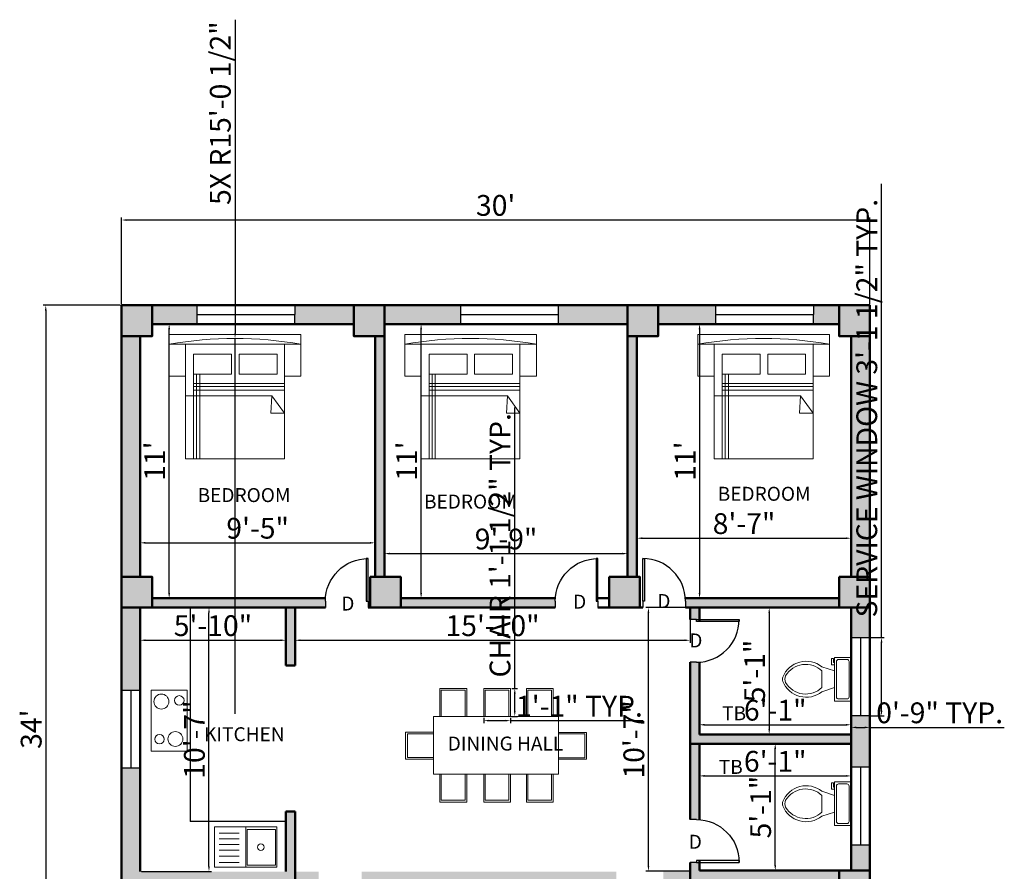
# Model space of a CAD drawing. Units: inches. Extents: x 1864 to 2337, y 2028 to 2650.
# Tile 2 of 2: x 1864 to 2337, y 2240 to 2650. Entities that reach past the tile are written whole.
import ezdxf

# ---------------------------------------------------------------- set-up
doc = ezdxf.new("R2010")
doc.units = ezdxf.units.IN
for name, color, linetype, lineweight in [('A-ANNO-TEXT', 7, 'Continuous', 25), ('A-AREA-IDEN', 7, 'Continuous', 25), ('A-COLS-PATT', 10, 'Continuous', 13), ('A-EQPM', 93, 'Continuous', 18), ('A-FLOR-CASE', 7, 'Continuous', 25), ('A-FLOR-FIXT', 93, 'Continuous', 18), ('A-WALL-PATT', 144, 'Continuous', 13), ('BED', 220, 'Continuous', 18), ('COLUMN', 10, 'Continuous', 50), ('DIM', 130, 'Continuous', 18), ('WALL', 7, 'Continuous', 50)]:
    doc.layers.add(name, color=color, linetype=linetype, lineweight=lineweight)
for name, color, linetype, lineweight, plot in [('DINING', 11, 'Continuous', 18, False), ('DOOR', 50, 'Continuous', 25, False), ('WINDOW', 244, 'Continuous', 25, False)]:
    doc.layers.add(name, color=color, linetype=linetype, lineweight=lineweight, plot=plot)
doc.styles.get("Standard").update_dxf_attribs({"font": 'arial.ttf'})
doc.dimstyles.new('ISO-25', dxfattribs={"dimtxt": 10, "dimasz": 2.5, "dimexe": 1.25, "dimexo": 0.625, "dimtad": 1, "dimdec": 0, "dimlunit": 4, "dimtxsty": 'Standard', "dimcen": 2.5, "dimadec": 0, "dimazin": 0, "dimtfac": 1, "dimtdec": 0, "dimtmove": 0, "dimatfit": 3, "dimfxl": 1, "dimarcsym": 0})

# ---------------------------------------------------------------- blocks, each defined once
blk = doc.blocks.new('*U4')
for p, q in [((9.5, -6), (9.5, -2)), ((-10, -8.5), (-8, -8.5)), ((-10, -9.5), (-10, -8.5)), ((-8, -8.5), (-8, -8)), ((-7, -8), (-7, -9.5)), ((-4, -8), (-6, -14)), ((4, -8), (6, -14)), ((-7, -9.5), (-10, -9.5)), ((4, -14), (-4, -14))]:
    blk.add_line(p, q)
blk.add_lwpolyline([(10.5, -8), (10.5, 0), (-10.5, 0), (-10.5, -8)], close=True)
for points in [[(-9.5, -2), (-9.5, -6)], [(8.5, -1), (-8.5, -1)], [(-8.5, -7), (8.5, -7)]]:
    blk.add_lwpolyline(points)
for centre, radius, start, end in [((-8.62, -1.88), 0.884, 81.8699, 188.1301), ((8.62, -1.88), 0.884, 351.8699, 98.1301), ((-8.62, -6.12), 0.884, 171.8699, 278.1301), ((8.62, -6.12), 0.884, 261.8699, 8.1301), ((3.52, -21.58), 12.17, 141.4691, 247.9714), ((4.2, -21.82), 11.33, 136.3677, 238.9468), ((-3.52, -21.58), 12.17, 292.0284, 38.5307), ((-4.2, -21.82), 11.33, 301.053, 43.6321), ((0, -27.88), 4, 245.7318, 294.2682), ((0, -29), 4, 254.8605, 285.1395)]:
    blk.add_arc(centre, radius, start, end)
blk = doc.blocks.new('*U2')
for p, q in [((0, 0), (0, -6)), ((40, 0), (40, -6))]:
    blk.add_line(p, q)
blk.add_lwpolyline([(0, 0), (0, 40), (1.75, 40), (1.75, 0)], close=True)
blk.add_arc((0, 0), 40, 0, 90)
blk = doc.blocks.new('*D5')
at = {"layer": 'Defpoints', "color": 0, "transparency": 16777216}
for p in [(1921.75, 2497.33), (2034.75, 2497.33), (2034.75, 2397.81)]:
    blk.add_point(p, dxfattribs=at)
at = {"layer": 'DIM', "color": 0, "lineweight": -2, "transparency": 16777216}
for p, q in [((1921.75, 2496.7), (1921.75, 2396.56)), ((2034.75, 2496.7), (2034.75, 2396.56)), ((1924.25, 2397.81), (2032.25, 2397.81))]:
    blk.add_line(p, q, dxfattribs=at)
at = {"layer": 'DIM', "color": 0, "transparency": 16777216}
for points in [[(1924.25, 2398.23), (1924.25, 2397.4), (1921.75, 2397.81)], [(2032.25, 2398.23), (2032.25, 2397.4), (2034.75, 2397.81)]]:
    blk.add_solid(points, dxfattribs=at)
at = {"layer": 'DIM', "color": 0, "transparency": 16777216, "insert": (1978.25, 2403.54), "char_height": 10, "attachment_point": 5}
blk.add_mtext('9\'-5"', dxfattribs=at)
blk = doc.blocks.new('*D6')
at = {"layer": 'Defpoints', "color": 0, "transparency": 16777216}
for p in [(1927.51, 2503.12), (1935.69, 2503.12), (1927.51, 2371.12)]:
    blk.add_point(p, dxfattribs=at)
at = {"layer": 'DIM', "color": 0, "lineweight": -2, "transparency": 16777216}
for p, q in [((1928.14, 2503.12), (1936.94, 2503.12)), ((1935.69, 2373.62), (1935.69, 2500.62)), ((1928.14, 2371.12), (1936.94, 2371.12))]:
    blk.add_line(p, q, dxfattribs=at)
at = {"layer": 'DIM', "color": 0, "transparency": 16777216}
for points in [[(1935.27, 2500.62), (1936.11, 2500.62), (1935.69, 2503.12)], [(1935.27, 2373.62), (1936.11, 2373.62), (1935.69, 2371.12)]]:
    blk.add_solid(points, dxfattribs=at)
at = {"layer": 'DIM', "color": 0, "transparency": 16777216, "insert": (1930.04, 2437.12), "char_height": 10, "attachment_point": 5, "rotation": 90}
blk.add_mtext("11'", dxfattribs=at)
blk = doc.blocks.new('*D7')
at = {"layer": 'Defpoints', "color": 0, "transparency": 16777216}
for p in [(2039.25, 2503.12), (2056.9, 2503.12), (2047.12, 2371.12)]:
    blk.add_point(p, dxfattribs=at)
at = {"layer": 'DIM', "color": 0, "lineweight": -2, "transparency": 16777216}
for p, q in [((2039.88, 2503.12), (2058.15, 2503.12)), ((2056.9, 2373.62), (2056.9, 2500.62)), ((2047.75, 2371.12), (2058.15, 2371.12))]:
    blk.add_line(p, q, dxfattribs=at)
at = {"layer": 'DIM', "color": 0, "transparency": 16777216}
for points in [[(2056.48, 2500.62), (2057.32, 2500.62), (2056.9, 2503.12)], [(2056.48, 2373.62), (2057.32, 2373.62), (2056.9, 2371.12)]]:
    blk.add_solid(points, dxfattribs=at)
at = {"layer": 'DIM', "color": 0, "transparency": 16777216, "insert": (2051.25, 2437.12), "char_height": 10, "attachment_point": 5, "rotation": 90}
blk.add_mtext("11'", dxfattribs=at)
blk = doc.blocks.new('*D8')
at = {"layer": 'Defpoints', "color": 0, "transparency": 16777216}
for p in [(2156.25, 2392.62), (2039.25, 2381.41), (2156.25, 2381.41)]:
    blk.add_point(p, dxfattribs=at)
at = {"layer": 'DIM', "color": 0, "lineweight": -2, "transparency": 16777216}
for p, q in [((2039.25, 2382.03), (2039.25, 2393.87)), ((2041.75, 2392.62), (2153.75, 2392.62)), ((2156.25, 2382.03), (2156.25, 2393.87))]:
    blk.add_line(p, q, dxfattribs=at)
at = {"layer": 'DIM', "color": 0, "transparency": 16777216}
for points in [[(2041.75, 2393.04), (2041.75, 2392.21), (2039.25, 2392.62)], [(2153.75, 2393.04), (2153.75, 2392.21), (2156.25, 2392.62)]]:
    blk.add_solid(points, dxfattribs=at)
at = {"layer": 'DIM', "color": 0, "transparency": 16777216, "insert": (2097.75, 2398.35), "char_height": 10, "attachment_point": 5}
blk.add_mtext('9\'-9"', dxfattribs=at)
blk = doc.blocks.new('*D9')
at = {"layer": 'Defpoints', "color": 0, "transparency": 16777216}
for p in [(2160.75, 2497.33), (2263.75, 2497.33), (2263.75, 2400.03)]:
    blk.add_point(p, dxfattribs=at)
at = {"layer": 'DIM', "color": 0, "lineweight": -2, "transparency": 16777216}
for p, q in [((2160.75, 2496.7), (2160.75, 2398.78)), ((2263.75, 2496.7), (2263.75, 2398.78)), ((2163.25, 2400.03), (2261.25, 2400.03))]:
    blk.add_line(p, q, dxfattribs=at)
at = {"layer": 'DIM', "color": 0, "transparency": 16777216}
for points in [[(2163.25, 2400.45), (2163.25, 2399.61), (2160.75, 2400.03)], [(2261.25, 2400.45), (2261.25, 2399.61), (2263.75, 2400.03)]]:
    blk.add_solid(points, dxfattribs=at)
at = {"layer": 'DIM', "color": 0, "transparency": 16777216, "insert": (2212.25, 2405.76), "char_height": 10, "attachment_point": 5}
blk.add_mtext('8\'-7"', dxfattribs=at)
blk = doc.blocks.new('*D10')
at = {"layer": 'Defpoints', "color": 0, "transparency": 16777216}
for p in [(2258, 2503.12), (2190.85, 2371.12), (2258, 2371.12)]:
    blk.add_point(p, dxfattribs=at)
at = {"layer": 'DIM', "color": 0, "lineweight": -2, "transparency": 16777216}
for p, q in [((2257.37, 2503.12), (2189.6, 2503.12)), ((2190.85, 2500.62), (2190.85, 2373.62)), ((2257.37, 2371.12), (2189.6, 2371.12))]:
    blk.add_line(p, q, dxfattribs=at)
at = {"layer": 'DIM', "color": 0, "transparency": 16777216}
for points in [[(2190.43, 2500.62), (2191.27, 2500.62), (2190.85, 2503.12)], [(2190.43, 2373.62), (2191.27, 2373.62), (2190.85, 2371.12)]]:
    blk.add_solid(points, dxfattribs=at)
at = {"layer": 'DIM', "color": 0, "transparency": 16777216, "insert": (2185.2, 2437.12), "char_height": 10, "attachment_point": 5, "rotation": 90}
blk.add_mtext("11'", dxfattribs=at)
blk = doc.blocks.new('*D11')
at = {"layer": 'Defpoints', "color": 0, "transparency": 16777216}
for p in [(2263.75, 2366.62), (2224.35, 2305.62), (2263.75, 2305.62)]:
    blk.add_point(p, dxfattribs=at)
at = {"layer": 'DIM', "color": 0, "lineweight": -2, "transparency": 16777216}
for p, q in [((2263.13, 2366.62), (2223.1, 2366.62)), ((2224.35, 2364.12), (2224.35, 2308.12)), ((2263.13, 2305.62), (2223.1, 2305.62))]:
    blk.add_line(p, q, dxfattribs=at)
at = {"layer": 'DIM', "color": 0, "transparency": 16777216}
for points in [[(2223.94, 2364.12), (2224.77, 2364.12), (2224.35, 2366.62)], [(2223.94, 2308.12), (2224.77, 2308.12), (2224.35, 2305.62)]]:
    blk.add_solid(points, dxfattribs=at)
at = {"layer": 'DIM', "color": 0, "transparency": 16777216, "insert": (2218.62, 2336.12), "char_height": 10, "attachment_point": 5, "rotation": 90}
blk.add_mtext('5\'-1"', dxfattribs=at)
blk = doc.blocks.new('*D12')
at = {"layer": 'Defpoints', "color": 0, "transparency": 16777216}
for p in [(2263.75, 2310.24), (2190.75, 2305.62), (2263.75, 2305.62)]:
    blk.add_point(p, dxfattribs=at)
at = {"layer": 'DIM', "color": 0, "lineweight": -2, "transparency": 16777216}
for p, q in [((2190.75, 2306.24), (2190.75, 2311.49)), ((2193.25, 2310.24), (2261.25, 2310.24)), ((2263.75, 2306.24), (2263.75, 2311.49))]:
    blk.add_line(p, q, dxfattribs=at)
at = {"layer": 'DIM', "color": 0, "transparency": 16777216}
for points in [[(2193.25, 2310.66), (2193.25, 2309.82), (2190.75, 2310.24)], [(2261.25, 2310.66), (2261.25, 2309.82), (2263.75, 2310.24)]]:
    blk.add_solid(points, dxfattribs=at)
at = {"layer": 'DIM', "color": 0, "transparency": 16777216, "insert": (2227.25, 2315.97), "char_height": 10, "attachment_point": 5}
blk.add_mtext('6\'-1"', dxfattribs=at)
blk = doc.blocks.new('*D13')
at = {"layer": 'Defpoints', "color": 0, "transparency": 16777216}
for p in [(2190.75, 2301.12), (2263.75, 2301.12), (2263.75, 2285.64)]:
    blk.add_point(p, dxfattribs=at)
at = {"layer": 'DIM', "color": 0, "lineweight": -2, "transparency": 16777216}
for p, q in [((2190.75, 2300.49), (2190.75, 2284.39)), ((2263.75, 2300.49), (2263.75, 2284.39)), ((2193.25, 2285.64), (2261.25, 2285.64))]:
    blk.add_line(p, q, dxfattribs=at)
at = {"layer": 'DIM', "color": 0, "transparency": 16777216}
for points in [[(2193.25, 2286.05), (2193.25, 2285.22), (2190.75, 2285.64)], [(2261.25, 2286.05), (2261.25, 2285.22), (2263.75, 2285.64)]]:
    blk.add_solid(points, dxfattribs=at)
at = {"layer": 'DIM', "color": 0, "transparency": 16777216, "insert": (2227.25, 2291.37), "char_height": 10, "attachment_point": 5}
blk.add_mtext('6\'-1"', dxfattribs=at)
blk = doc.blocks.new('*D14')
at = {"layer": 'Defpoints', "color": 0, "transparency": 16777216}
for p in [(2227.25, 2301.12), (2263.75, 2301.12), (2263.75, 2240.12)]:
    blk.add_point(p, dxfattribs=at)
at = {"layer": 'DIM', "color": 0, "lineweight": -2, "transparency": 16777216}
for p, q in [((2263.13, 2301.12), (2226, 2301.12)), ((2227.25, 2242.62), (2227.25, 2298.62)), ((2263.13, 2240.12), (2226, 2240.12))]:
    blk.add_line(p, q, dxfattribs=at)
at = {"layer": 'DIM', "color": 0, "transparency": 16777216}
for points in [[(2226.84, 2298.62), (2227.67, 2298.62), (2227.25, 2301.12)], [(2226.84, 2242.62), (2227.67, 2242.62), (2227.25, 2240.12)]]:
    blk.add_solid(points, dxfattribs=at)
at = {"layer": 'DIM', "color": 0, "transparency": 16777216, "insert": (2221.52, 2270.62), "char_height": 10, "attachment_point": 5, "rotation": 90}
blk.add_mtext('5\'-1"', dxfattribs=at)
blk = doc.blocks.new('*D15')
at = {"layer": 'Defpoints', "color": 0, "transparency": 16777216}
for p in [(1996.25, 2366.62), (2186.25, 2366.62), (2186.25, 2350.91)]:
    blk.add_point(p, dxfattribs=at)
at = {"layer": 'DIM', "color": 0, "lineweight": -2, "transparency": 16777216}
for p, q in [((1996.25, 2365.99), (1996.25, 2349.66)), ((2186.25, 2365.99), (2186.25, 2349.66)), ((1998.75, 2350.91), (2183.75, 2350.91))]:
    blk.add_line(p, q, dxfattribs=at)
at = {"layer": 'DIM', "color": 0, "transparency": 16777216}
for points in [[(1998.75, 2351.33), (1998.75, 2350.5), (1996.25, 2350.91)], [(2183.75, 2351.33), (2183.75, 2350.5), (2186.25, 2350.91)]]:
    blk.add_solid(points, dxfattribs=at)
at = {"layer": 'DIM', "color": 0, "transparency": 16777216, "insert": (2091.25, 2356.64), "char_height": 10, "attachment_point": 5}
blk.add_mtext('15\'-10"', dxfattribs=at)
blk = doc.blocks.new('*D16')
at = {"layer": 'Defpoints', "color": 0, "transparency": 16777216}
for p in [(2166.25, 2366.62), (2186.25, 2366.62), (2186.25, 2239.82)]:
    blk.add_point(p, dxfattribs=at)
at = {"layer": 'DIM', "color": 0, "lineweight": -2, "transparency": 16777216}
for p, q in [((2185.63, 2366.62), (2165, 2366.62)), ((2166.25, 2242.32), (2166.25, 2364.12)), ((2185.63, 2239.82), (2165, 2239.82))]:
    blk.add_line(p, q, dxfattribs=at)
at = {"layer": 'DIM', "color": 0, "transparency": 16777216}
for points in [[(2165.84, 2364.12), (2166.67, 2364.12), (2166.25, 2366.62)], [(2165.84, 2242.32), (2166.67, 2242.32), (2166.25, 2239.82)]]:
    blk.add_solid(points, dxfattribs=at)
at = {"layer": 'DIM', "color": 0, "transparency": 16777216, "insert": (2160.52, 2303.22), "char_height": 10, "attachment_point": 5, "rotation": 90}
blk.add_mtext('10\'-7"', dxfattribs=at)
blk = doc.blocks.new('*D17')
at = {"layer": 'Defpoints', "color": 0, "transparency": 16777216}
for p in [(1921.75, 2366.62), (1991.75, 2366.62), (1991.75, 2350.92)]:
    blk.add_point(p, dxfattribs=at)
at = {"layer": 'DIM', "color": 0, "lineweight": -2, "transparency": 16777216}
for p, q in [((1921.75, 2365.99), (1921.75, 2349.67)), ((1991.75, 2365.99), (1991.75, 2349.67)), ((1924.25, 2350.92), (1989.25, 2350.92))]:
    blk.add_line(p, q, dxfattribs=at)
at = {"layer": 'DIM', "color": 0, "transparency": 16777216}
for points in [[(1924.25, 2351.34), (1924.25, 2350.51), (1921.75, 2350.92)], [(1989.25, 2351.34), (1989.25, 2350.51), (1991.75, 2350.92)]]:
    blk.add_solid(points, dxfattribs=at)
at = {"layer": 'DIM', "color": 0, "transparency": 16777216, "insert": (1956.75, 2356.65), "char_height": 10, "attachment_point": 5}
blk.add_mtext('5\'-10"', dxfattribs=at)
blk = doc.blocks.new('*D18')
at = {"layer": 'Defpoints', "color": 0, "transparency": 16777216}
for p in [(1921.75, 2366.62), (1954.84, 2366.62), (1921.75, 2239.62)]:
    blk.add_point(p, dxfattribs=at)
at = {"layer": 'DIM', "color": 0, "lineweight": -2, "transparency": 16777216}
for p, q in [((1922.38, 2366.62), (1956.09, 2366.62)), ((1954.84, 2242.12), (1954.84, 2364.12)), ((1922.38, 2239.62), (1956.09, 2239.62))]:
    blk.add_line(p, q, dxfattribs=at)
at = {"layer": 'DIM', "color": 0, "transparency": 16777216}
for points in [[(1954.42, 2364.12), (1955.25, 2364.12), (1954.84, 2366.62)], [(1954.42, 2242.12), (1955.25, 2242.12), (1954.84, 2239.62)]]:
    blk.add_solid(points, dxfattribs=at)
at = {"layer": 'DIM', "color": 0, "transparency": 16777216, "insert": (1949.11, 2303.12), "char_height": 10, "attachment_point": 5, "rotation": 90}
blk.add_mtext('10\'-7"', dxfattribs=at)
blk = doc.blocks.new('*D25')
at = {"layer": 'Defpoints', "color": 0, "transparency": 16777216}
for p in [(2272.75, 2553.18), (1912.75, 2512.12), (2272.75, 2512.12)]:
    blk.add_point(p, dxfattribs=at)
at = {"layer": 'DIM', "color": 0, "lineweight": -2, "transparency": 16777216}
for p, q in [((1912.75, 2512.74), (1912.75, 2554.43)), ((2272.75, 2512.74), (2272.75, 2554.43)), ((1915.25, 2553.18), (2270.25, 2553.18))]:
    blk.add_line(p, q, dxfattribs=at)
at = {"layer": 'DIM', "color": 0, "transparency": 16777216}
for points in [[(1915.25, 2553.59), (1915.25, 2552.76), (1912.75, 2553.18)], [(2270.25, 2553.59), (2270.25, 2552.76), (2272.75, 2553.18)]]:
    blk.add_solid(points, dxfattribs=at)
at = {"layer": 'DIM', "color": 0, "transparency": 16777216, "insert": (2092.75, 2558.91), "char_height": 10, "attachment_point": 5}
blk.add_mtext("30'", dxfattribs=at)
blk = doc.blocks.new('*D26')
at = {"layer": 'Defpoints', "color": 0, "transparency": 16777216}
for p in [(1912.75, 2512.12), (1876.32, 2104.12), (1912.75, 2104.12)]:
    blk.add_point(p, dxfattribs=at)
at = {"layer": 'DIM', "color": 0, "lineweight": -2, "transparency": 16777216}
for p, q in [((1912.13, 2512.12), (1875.07, 2512.12)), ((1876.32, 2509.62), (1876.32, 2106.62)), ((1912.13, 2104.12), (1875.07, 2104.12))]:
    blk.add_line(p, q, dxfattribs=at)
at = {"layer": 'DIM', "color": 0, "transparency": 16777216}
for points in [[(1875.9, 2509.62), (1876.74, 2509.62), (1876.32, 2512.12)], [(1875.9, 2106.62), (1876.74, 2106.62), (1876.32, 2104.12)]]:
    blk.add_solid(points, dxfattribs=at)
at = {"layer": 'DIM', "color": 0, "transparency": 16777216, "insert": (1870.59, 2308.12), "char_height": 10, "attachment_point": 5, "rotation": 90}
blk.add_mtext("34'", dxfattribs=at)
blk = doc.blocks.new('BED-DOUBLE')
for p, q in [((11.74, 40.81), (11.74, 0)), ((13.19, 40.81), (13.19, 0)), ((14.75, 40.81), (14.75, 0)), ((11.74, 36.25), (55.45, 36.25)), ((11.74, 34.82), (55.45, 34.82)), ((7.92, 30.28), (49.44, 30.28)), ((11.74, 33.07), (55.45, 33.07)), ((48.97, 21.97), (49.44, 30.28)), ((49.44, 30.28), (55.45, 21.97)), ((55.45, 21.97), (48.97, 21.97))]:
    blk.add_line(p, q)
for points in [[(0, 55.15), (63.37, 55.15), (63.37, 59.81), (0, 59.81)], [(7.92, 55.15), (0, 55.15), (0, 39.81), (7.92, 39.81)], [(7.92, 55.15), (55.45, 55.15), (55.45, 0), (7.92, 0)], [(63.37, 55.15), (55.45, 55.15), (55.45, 39.81), (63.37, 39.81)], [(11.74, 50.29), (29.99, 50.29), (29.99, 40.81), (11.74, 40.81)], [(33.64, 50.29), (51.9, 50.29), (51.9, 40.81), (33.64, 40.81)]]:
    blk.add_lwpolyline(points, close=True)
blk.add_arc((31.69, -122.73), 180.68, 79.9001, 100.0999)
blk = doc.blocks.new('CHAIR-DINING')
for points in [[(0, 0), (12.9, 0), (12.9, 13.49), (0, 13.49)], [(0.68, 0), (12.12, 0), (12.12, 12.58), (0.68, 12.58)]]:
    blk.add_lwpolyline(points, close=True)
blk = doc.blocks.new('WIN-BEDROOM')
blk.add_line((0.02, 4.5), (46.93, 4.5))
blk.add_lwpolyline([(0.04, 9), (46.95, 9), (46.91, 0), (0, 0)], close=True)
blk = doc.blocks.new('WIN-SERVICE')
blk.add_line((4.5, 37.59), (4.5, 0))
blk.add_lwpolyline([(0, 37.59), (9, 37.59), (9, 0), (0, 0)], close=True)
blk = doc.blocks.new('*D35')
at = {"layer": 'Defpoints', "color": 0, "transparency": 16777216}
for p in [(2272.75, 2352.2), (2278.39, 2352.2), (2272.75, 2314.61)]:
    blk.add_point(p, dxfattribs=at)
at = {"layer": 'DIM', "color": 0, "lineweight": -2, "transparency": 16777216}
for p, q in [((2278.39, 2352.2), (2278.39, 2570.54)), ((2273.38, 2352.2), (2279.64, 2352.2)), ((2278.39, 2317.11), (2278.39, 2349.7)), ((2273.38, 2314.61), (2279.64, 2314.61))]:
    blk.add_line(p, q, dxfattribs=at)
at = {"layer": 'DIM', "color": 0, "transparency": 16777216}
for points in [[(2277.98, 2349.7), (2278.81, 2349.7), (2278.39, 2352.2)], [(2277.98, 2317.11), (2278.81, 2317.11), (2278.39, 2314.61)]]:
    blk.add_solid(points, dxfattribs=at)
at = {"layer": 'DIM', "color": 0, "transparency": 16777216, "insert": (2272.59, 2462.62), "char_height": 10, "attachment_point": 5, "rotation": 90}
blk.add_mtext('SERVICE WINDOW 3\'-1 1/2" TYP.', dxfattribs=at)
blk = doc.blocks.new('*D36')
at = {"layer": 'Defpoints', "color": 0, "transparency": 16777216}
for p in [(2263.75, 2314.61), (2272.75, 2314.61), (2272.75, 2308.97)]:
    blk.add_point(p, dxfattribs=at)
at = {"layer": 'DIM', "color": 0, "lineweight": -2, "transparency": 16777216}
for p, q in [((2263.75, 2313.98), (2263.75, 2307.72)), ((2272.75, 2313.98), (2272.75, 2307.72)), ((2266.25, 2308.97), (2270.25, 2308.97)), ((2272.75, 2308.97), (2337.46, 2308.97))]:
    blk.add_line(p, q, dxfattribs=at)
at = {"layer": 'DIM', "color": 0, "transparency": 16777216}
for points in [[(2266.25, 2309.39), (2266.25, 2308.55), (2263.75, 2308.97)], [(2270.25, 2309.39), (2270.25, 2308.55), (2272.75, 2308.97)]]:
    blk.add_solid(points, dxfattribs=at)
at = {"layer": 'DIM', "color": 0, "transparency": 16777216, "insert": (2306.36, 2314.7), "char_height": 10, "attachment_point": 5}
blk.add_mtext('0\'-9" TYP.', dxfattribs=at)
blk = doc.blocks.new('*D37')
at = {"layer": 'Defpoints', "color": 0, "transparency": 16777216}
for p in [(2099.93, 2327.74), (2101.95, 2327.74), (2099.93, 2314.26)]:
    blk.add_point(p, dxfattribs=at)
at = {"layer": 'DIM', "color": 0, "lineweight": -2, "transparency": 16777216}
for p, q in [((2101.95, 2327.74), (2101.95, 2462.98)), ((2100.55, 2327.74), (2103.2, 2327.74)), ((2101.95, 2316.76), (2101.95, 2325.24)), ((2100.55, 2314.26), (2103.2, 2314.26))]:
    blk.add_line(p, q, dxfattribs=at)
at = {"layer": 'DIM', "color": 0, "transparency": 16777216}
for points in [[(2101.53, 2325.24), (2102.37, 2325.24), (2101.95, 2327.74)], [(2101.53, 2316.76), (2102.37, 2316.76), (2101.95, 2314.26)]]:
    blk.add_solid(points, dxfattribs=at)
at = {"layer": 'DIM', "color": 0, "transparency": 16777216, "insert": (2096.15, 2396.61), "char_height": 10, "attachment_point": 5, "rotation": 90}
blk.add_mtext('CHAIR 1\'-1 1/2" TYP.', dxfattribs=at)
blk = doc.blocks.new('*D38')
at = {"layer": 'Defpoints', "color": 0, "transparency": 16777216}
for p in [(2087.03, 2314.26), (2099.93, 2314.26), (2099.93, 2312.23)]:
    blk.add_point(p, dxfattribs=at)
at = {"layer": 'DIM', "color": 0, "lineweight": -2, "transparency": 16777216}
for p, q in [((2087.03, 2313.63), (2087.03, 2310.98)), ((2089.53, 2312.23), (2097.43, 2312.23)), ((2099.93, 2313.63), (2099.93, 2310.98)), ((2099.93, 2312.23), (2163.69, 2312.23))]:
    blk.add_line(p, q, dxfattribs=at)
at = {"layer": 'DIM', "color": 0, "transparency": 16777216}
for points in [[(2089.53, 2312.65), (2089.53, 2311.82), (2087.03, 2312.23)], [(2097.43, 2312.65), (2097.43, 2311.82), (2099.93, 2312.23)]]:
    blk.add_solid(points, dxfattribs=at)
at = {"layer": 'DIM', "color": 0, "transparency": 16777216, "insert": (2133.06, 2317.88), "char_height": 10, "attachment_point": 5}
blk.add_mtext('1\'-1" TYP.', dxfattribs=at)
blk = doc.blocks.new('*D39')
at = {"layer": 'Defpoints', "color": 0, "transparency": 16777216}
for p in [(1967.37, 2496.2), (1967.37, 2315.51)]:
    blk.add_point(p, dxfattribs=at)
at = {"layer": 'DIM', "color": 0, "lineweight": -2, "transparency": 16777216}
for p, q in [((1967.37, 2649.59), (1967.37, 2498.7)), ((1967.37, 2315.51), (1967.37, 2496.2))]:
    blk.add_line(p, q, dxfattribs=at)
at = {"layer": 'DIM', "color": 0, "transparency": 16777216}
blk.add_solid([(1966.96, 2498.7), (1967.79, 2498.7), (1967.37, 2496.2)], dxfattribs=at)
at = {"layer": 'DIM', "color": 0, "transparency": 16777216, "insert": (1961.58, 2604.61), "char_height": 10, "attachment_point": 5, "rotation": 90}
blk.add_mtext('5X R15\'-0 1/2"', dxfattribs=at)

msp = doc.modelspace()

# ---------------------------------------------------------------- hatches: boundary and pattern name
at = {"layer": 'A-COLS-PATT'}
h = msp.add_hatch(color=256, dxfattribs=at)
h.dxf.hatch_style = 1
h.paths.add_polyline_path([(1927.51, 2512.12), (1912.75, 2512.12), (1912.75, 2497.33), (1927.51, 2497.33)])
h.paths.add_polyline_path([(2039.25, 2512.12), (2024.5, 2512.12), (2024.5, 2497.35), (2039.25, 2497.35)])
h.paths.add_polyline_path([(2049.51, 2239.62), (2034.75, 2239.62), (2034.75, 2224.83), (2049.51, 2224.83)])
h.paths.add_polyline_path([(2150.75, 2239.62), (2136, 2239.62), (2136, 2224.83), (2150.75, 2224.83)])
h.paths.add_polyline_path([(2272.75, 2240.1), (2258, 2240.1), (2258, 2225.31), (2272.75, 2225.31)])
h.paths.add_polyline_path([(2272.75, 2118.91), (2258, 2118.91), (2258, 2104.12), (2272.75, 2104.12)])
h.paths.add_polyline_path([(2161.01, 2118.91), (2146.25, 2118.91), (2146.25, 2104.12), (2161.01, 2104.12)])
h.paths.add_polyline_path([(2049.47, 2118.91), (2034.75, 2118.91), (2034.75, 2113.12), (2034.71, 2104.12), (2049.47, 2104.12)])
h.paths.add_polyline_path([(1927.51, 2118.91), (1912.75, 2118.91), (1912.75, 2104.12), (1927.51, 2104.12)])
h.paths.add_polyline_path([(1927.51, 2239.62), (1912.75, 2239.62), (1912.75, 2224.83), (1927.51, 2224.83)])
h.paths.add_polyline_path([(1927.51, 2381.41), (1912.75, 2381.41), (1912.75, 2366.62), (1927.51, 2366.62)])
h.paths.add_polyline_path([(2272.75, 2512.12), (2258, 2512.12), (2258, 2497.33), (2272.75, 2497.33)])
h.paths.add_polyline_path([(2170.98, 2512.12), (2156.22, 2512.12), (2156.22, 2503.12), (2156.25, 2503.12), (2156.25, 2497.33), (2170.98, 2497.33)])
h = msp.add_hatch(color=256, dxfattribs=at)
h.dxf.hatch_style = 1
h.paths.add_polyline_path([(2047.12, 2381.41), (2032.36, 2381.41), (2032.36, 2366.62), (2047.12, 2366.62)])
h.paths.add_polyline_path([(2162.13, 2381.41), (2147.37, 2381.41), (2147.37, 2366.62), (2162.13, 2366.62)])
h.paths.add_polyline_path([(2272.75, 2381.41), (2258, 2381.41), (2258, 2366.62), (2272.75, 2366.62)])
at = {"layer": 'A-WALL-PATT'}
h = msp.add_hatch(color=256, dxfattribs=at)
h.dxf.hatch_style = 1
h.paths.add_polyline_path([(1921.75, 2224.83), (1912.75, 2224.83), (1912.75, 2118.91), (1921.75, 2118.91)])
h.paths.add_polyline_path([(2039.25, 2224.83), (2034.75, 2224.83), (2034.75, 2118.91), (2039.25, 2118.91)])
h.paths.add_polyline_path([(2150.75, 2224.83), (2146.25, 2224.83), (2146.25, 2118.91), (2150.75, 2118.91)])
h.paths.add_polyline_path([(2272.75, 2225.31), (2263.75, 2225.31), (2263.75, 2118.91), (2272.75, 2118.91)])
h.paths.add_polyline_path([(2258, 2240.12), (2190.75, 2240.12), (2190.75, 2244.03), (2189.34, 2244.03), (2186.25, 2244.03), (2186.25, 2235.62), (2186.25, 2235.12), (2228.41, 2235.12), (2258, 2235.12)])
h.paths.add_polyline_path([(2190.75, 2301.12), (2186.25, 2301.12), (2186.25, 2264.6), (2189.34, 2264.6, -0.017198), (2190.75, 2264.55)])
h.paths.add_polyline_path([(2136, 2239.62), (2049.51, 2239.62), (2049.51, 2235.12), (2136, 2235.12)])
h.paths.add_polyline_path([(2186.25, 2239.62), (2173.41, 2239.62), (2173.41, 2236.53, -0.017198), (2173.36, 2235.12), (2186.25, 2235.12), (2186.25, 2235.62)])
h.paths.add_polyline_path([(1996.25, 2239.62), (1991.75, 2239.62), (1927.51, 2239.62), (1927.51, 2235.12), (1996.25, 2235.12)])
h.paths.add_polyline_path([(2007.65, 2239.62), (1996.25, 2239.62), (1996.25, 2235.12), (2007.7, 2235.12, -0.017198), (2007.65, 2236.53)])
h.paths.add_polyline_path([(2010.85, 2369.7, -0.017198), (2010.89, 2371.12), (1927.51, 2371.12), (1927.51, 2366.62), (2010.85, 2366.62)])
h.paths.add_polyline_path([(1996.25, 2366.62), (1991.75, 2366.62), (1991.75, 2338.77), (1996.25, 2338.77)])
h.paths.add_polyline_path([(2121.41, 2369.7, -0.017198), (2121.46, 2371.12), (2047.12, 2371.12), (2047.12, 2366.62), (2121.41, 2366.62)])
h.paths.add_polyline_path([(2258, 2371.12), (2184.04, 2371.12, -0.017198), (2184.09, 2369.7), (2184.09, 2366.62), (2258, 2366.62)])
h.paths.add_polyline_path([(2190.75, 2366.62), (2186.25, 2366.62), (2186.25, 2360.91), (2189.34, 2360.91), (2190.75, 2360.91)])
h.paths.add_polyline_path([(2190.75, 2340.39, -0.017198), (2189.34, 2340.34), (2186.25, 2340.34), (2186.25, 2301.12), (2190.75, 2301.12), (2263.75, 2301.12), (2263.75, 2305.62), (2190.75, 2305.62)])
h.paths.add_polyline_path([(2272.75, 2497.33), (2263.75, 2497.33), (2263.75, 2381.41), (2272.75, 2381.41)])
h.paths.add_polyline_path([(2160.75, 2497.33), (2156.25, 2497.33), (2156.25, 2381.41), (2160.75, 2381.41)])
h.paths.add_polyline_path([(2039.25, 2497.35), (2034.75, 2497.35), (2034.75, 2381.41), (2039.25, 2381.41)])
h.paths.add_polyline_path([(1921.75, 2497.33), (1912.75, 2497.33), (1912.75, 2381.41), (1921.75, 2381.41)])
h.paths.add_polyline_path([(2111.85, 2104.12), (2111.85, 2106.36), (2112.5, 2106.36), (2112.5, 2113.12), (2049.47, 2113.12), (2049.47, 2104.12)])
h.paths.add_polyline_path([(2141.1, 2113.12), (2141.1, 2106.36), (2141.75, 2106.36), (2141.75, 2104.12), (2146.25, 2104.12), (2146.25, 2113.12)])
h.paths.add_polyline_path([(1996.08, 2512.12), (1996.04, 2503.12), (2024.5, 2503.12), (2024.5, 2512.12)])
h.paths.add_polyline_path([(1949.13, 2503.12), (1949.17, 2512.12), (1927.51, 2512.12), (1927.51, 2503.12)])
h.paths.add_polyline_path([(2122.88, 2512.12), (2122.84, 2503.12), (2156.22, 2503.12), (2156.22, 2512.12)])
h.paths.add_polyline_path([(2075.93, 2503.12), (2075.97, 2512.12), (2039.25, 2512.12), (2039.25, 2503.12)])
h.paths.add_polyline_path([(2245.62, 2512.12), (2245.58, 2503.12), (2258, 2503.12), (2258, 2512.12)])
h.paths.add_polyline_path([(2198.67, 2503.12), (2198.71, 2512.12), (2170.98, 2512.12), (2170.98, 2503.12)])
h.paths.add_polyline_path([(2263.75, 2352.2), (2272.75, 2352.2), (2272.75, 2366.62), (2263.75, 2366.62)])
h.paths.add_polyline_path([(2272.75, 2252.38), (2263.75, 2252.38), (2263.75, 2240.1), (2272.75, 2240.1)])
h.paths.add_polyline_path([(2263.75, 2289.97), (2272.75, 2289.97), (2272.75, 2314.61), (2263.75, 2314.61)])
h.paths.add_polyline_path([(2197.66, 2104.12), (2197.7, 2113.12), (2161.01, 2113.12), (2161.01, 2104.12)])
h.paths.add_polyline_path([(2244.61, 2113.12), (2244.57, 2104.12), (2258, 2104.12), (2258, 2113.12)])
h.paths.add_polyline_path([(1956.19, 2104.12), (1956.23, 2113.12), (1927.51, 2113.12), (1927.51, 2104.12)])
h.paths.add_polyline_path([(2003.14, 2113.12), (2003.1, 2104.12), (2034.71, 2104.12), (2034.71, 2113.12)])
h.paths.add_polyline_path([(1921.75, 2289.34), (1912.75, 2289.34), (1912.75, 2239.62), (1921.75, 2239.62)])
h.paths.add_polyline_path([(1912.75, 2326.93), (1921.75, 2326.93), (1921.75, 2366.62), (1912.75, 2366.62)])
h = msp.add_hatch(color=256, dxfattribs=at)
h.dxf.hatch_style = 1
h.paths.add_polyline_path([(2034.75, 2239.62), (2028.22, 2239.62), (2028.22, 2236.53), (2028.22, 2235.12), (2034.75, 2235.12)])
h.paths.add_polyline_path([(1996.25, 2268.5), (1991.75, 2268.5), (1991.75, 2239.62), (1996.25, 2239.62)])

# ---------------------------------------------------------------- linework, layer by layer
at = {"layer": 'A-EQPM'}
msp.add_lwpolyline([(1926.99, 2297.57), (1944.29, 2297.57), (1944.29, 2326.97), (1926.99, 2326.97)], close=True, dxfattribs=at)
for centre, radius in [((1931.94, 2321.42), 3.6), ((1940.54, 2321.97), 2.3), ((1938.69, 2303.4), 3.6), ((1931.02, 2303.3), 2.3)]:
    msp.add_circle(centre, radius, dxfattribs=at)
at = {"layer": 'A-FLOR-CASE'}
for p, q in [((1921.75, 2366.62), (1945.75, 2366.62)), ((1945.75, 2366.62), (1945.75, 2263.62)), ((1991.75, 2263.62), (1945.75, 2263.62)), ((1991.75, 2239.62), (1991.75, 2263.62))]:
    msp.add_line(p, q, dxfattribs=at)
at = {"layer": 'A-FLOR-FIXT'}
for p, q in [((1972.52, 2261.09), (1972.52, 2241.7)), ((1959.71, 2258.1), (1969.35, 2258.1)), ((1959.71, 2255.43), (1969.35, 2255.43)), ((1959.71, 2252.59), (1969.35, 2252.59)), ((1959.71, 2249.86), (1969.35, 2249.86)), ((1959.71, 2246.96), (1969.35, 2246.96)), ((1959.71, 2243.89), (1969.35, 2243.89))]:
    msp.add_line(p, q, dxfattribs=at)
for points in [[(1957.57, 2261.09), (1987.48, 2261.09), (1987.48, 2241.7), (1957.57, 2241.7)], [(1973.27, 2259.89), (1986.89, 2259.89), (1986.89, 2242.75), (1973.27, 2242.75)]]:
    msp.add_lwpolyline(points, close=True, dxfattribs=at)
msp.add_circle((1979.76, 2251.37), 1.58, dxfattribs=at)
at = {"layer": 'COLUMN'}
for points in [[(1912.75, 2512.12), (1927.51, 2512.12), (1927.51, 2497.33), (1912.75, 2497.33)], [(2024.5, 2512.14), (2039.25, 2512.14), (2039.25, 2497.35), (2024.5, 2497.35)], [(2156.22, 2512.12), (2170.98, 2512.12), (2170.98, 2497.33), (2156.22, 2497.33)], [(2258, 2512.12), (2272.75, 2512.12), (2272.75, 2497.33), (2258, 2497.33)], [(1912.75, 2381.41), (1927.51, 2381.41), (1927.51, 2366.62), (1912.75, 2366.62)], [(2032.36, 2381.41), (2047.12, 2381.41), (2047.12, 2366.62), (2032.36, 2366.62)], [(2147.37, 2381.41), (2162.13, 2381.41), (2162.13, 2366.62), (2147.37, 2366.62)], [(2258, 2381.41), (2272.76, 2381.41), (2272.76, 2366.62), (2258, 2366.62)], [(2258, 2240.1), (2272.75, 2240.1), (2272.75, 2225.31), (2258, 2225.31)]]:
    msp.add_lwpolyline(points, close=True, dxfattribs=at)
at = {"layer": 'DINING'}
msp.add_lwpolyline([(2062.91, 2314.26), (2123.01, 2314.26), (2123.01, 2286.48), (2062.91, 2286.48)], close=True, dxfattribs=at)
at = {"layer": 'WALL'}
for p, q in [((1927.51, 2503.12), (2024.5, 2503.12)), ((2039.25, 2503.12), (2039.25, 2381.41)), ((2039.25, 2503.12), (2156.25, 2503.12)), ((2156.25, 2503.12), (2156.25, 2381.41)), ((2256.32, 2503.12), (2258, 2503.12)), ((2034.75, 2497.35), (2034.75, 2381.41)), ((2160.75, 2497.33), (2160.75, 2381.41)), ((2010.89, 2371.12), (1927.51, 2371.12)), ((2121.46, 2371.12), (2047.12, 2371.12)), ((2141.08, 2371.12), (2147.37, 2371.12)), ((2184.04, 2371.12), (2258, 2371.12)), ((1921.75, 2366.62), (1991.75, 2366.62)), ((2010.85, 2366.62), (1921.75, 2366.62)), ((1991.75, 2366.62), (1991.75, 2338.77)), ((1996.25, 2366.62), (1996.25, 2338.77)), ((2039.25, 2366.62), (2031.42, 2366.62)), ((2121.41, 2366.62), (2039.25, 2366.62)), ((2141.98, 2366.62), (2154.24, 2366.62)), ((2160.75, 2366.62), (2154.24, 2366.62)), ((2160.75, 2366.62), (2163.51, 2366.62)), ((2184.09, 2366.62), (2263.75, 2366.62)), ((2186.25, 2366.62), (2186.25, 2360.91)), ((2263.75, 2366.62), (2190.75, 2366.62)), ((2190.75, 2366.62), (2190.75, 2360.01)), ((2186.25, 2340.34), (2186.25, 2301.12)), ((2190.75, 2340.39), (2190.75, 2305.62)), ((1991.75, 2338.77), (1996.25, 2338.77)), ((2190.75, 2305.62), (2263.75, 2305.62)), ((2186.25, 2301.12), (2263.75, 2301.12)), ((2186.25, 2264.6), (2186.25, 2301.12)), ((2190.75, 2264.55), (2190.75, 2301.12)), ((2263.75, 2301.12), (2263.75, 2240.12)), ((1991.75, 2268.5), (1996.25, 2268.5)), ((1991.75, 2268.5), (1991.75, 2239.62)), ((1996.25, 2268.5), (1996.25, 2235.12)), ((2186.25, 2235.62), (2186.25, 2244.03)), ((2190.75, 2240.12), (2190.75, 2244.93)), ((2263.75, 2240.12), (2190.75, 2240.12))]:
    msp.add_line(p, q, dxfattribs=at)
for points in [[(2141.75, 2104.12), (2272.75, 2104.12), (2272.75, 2512.12), (1912.75, 2512.12), (1912.75, 2104.12), (2111.85, 2104.12)], [(2024.5, 2503.12), (1927.51, 2503.12)], [(2156.25, 2503.12), (2039.25, 2503.12)], [(2257.88, 2503.12), (2170.98, 2503.12)], [(1921.75, 2497.33), (1921.75, 2381.41)], [(2263.75, 2381.41), (2263.75, 2497.33)], [(1921.75, 2366.62), (1921.75, 2239.62)], [(2263.75, 2240.1), (2263.75, 2366.62)]]:
    msp.add_lwpolyline(points, dxfattribs=at)

# ---------------------------------------------------------------- block references
at = {"layer": 'A-FLOR-FIXT', "rotation": 270}
for p in [(2263.75, 2332.16), (2263.75, 2272.25)]:
    msp.add_blockref('*U4', p, dxfattribs=at)
at = {"layer": 'BED'}
for p in [(1935.69, 2438.24), (2048.98, 2438.24), (2189.99, 2438.24)]:
    msp.add_blockref('BED-DOUBLE', p, dxfattribs=at)
at = {"layer": 'DINING'}
for p in [(2065.93, 2314.26), (2087.03, 2314.26), (2107.53, 2314.26)]:
    msp.add_blockref('CHAIR-DINING', p, dxfattribs=at)
at = {"layer": 'DINING', "extrusion": (0, 0, -1), "zscale": -1}
for p, rotation in [((-2062.91, 2306.63), 270.0000000000031), ((-2065.93, 2286.48), 180), ((-2087.03, 2286.48), 180), ((-2107.53, 2286.48), 180)]:
    msp.add_blockref('CHAIR-DINING', p, dxfattribs=dict(at, rotation=rotation))
at = {"layer": 'DINING', "rotation": 270.0000000000031}
msp.add_blockref('CHAIR-DINING', (2123.01, 2306.53), dxfattribs=at)
at = {"layer": 'DOOR', "yscale": 0.514332689134197, "zscale": 0.514332689134197}
for p, xscale in [((2031.42, 2369.7), -0.514332689134197), ((2141.98, 2369.7), -0.514332689134197), ((2163.51, 2369.7), 0.514332689134197)]:
    msp.add_blockref('*U2', p, dxfattribs=dict(at, xscale=xscale))
at = {"layer": 'DOOR', "yscale": 0.514332689134197, "zscale": 0.514332689134197, "rotation": 270}
for p, xscale in [((2189.34, 2360.91), 0.514332689134197), ((2189.34, 2244.03), -0.514332689134197)]:
    msp.add_blockref('*U2', p, dxfattribs=dict(at, xscale=xscale))
at = {"layer": 'WINDOW'}
for name, p in [('WIN-BEDROOM', (1949.13, 2503.12)), ('WIN-BEDROOM', (2075.93, 2503.12)), ('WIN-BEDROOM', (2198.67, 2503.12)), ('WIN-SERVICE', (2263.75, 2314.61)), ('WIN-SERVICE', (1912.76, 2289.34)), ('WIN-SERVICE', (2263.75, 2252.38))]:
    msp.add_blockref(name, p, dxfattribs=at)

# ---------------------------------------------------------------- texts
at = {"layer": 'A-ANNO-TEXT', "char_height": 6.73, "attachment_point": 1}
for insert in [(2018.48, 2371.96), (2130.01, 2372.85), (2170.54, 2373.15), (2185.9, 2354.18), (2185.65, 2257.29)]:
    msp.add_mtext_dynamic_manual_height_columns('D', width=141.616, gutter_width=33.65, heights=[0], dxfattribs=dict(at, insert=insert))
at = {"layer": 'A-AREA-IDEN', "attachment_point": 1}
for s, insert, char_height in [('BEDROOM', (1949.36, 2424.15), 6.73), ('BEDROOM', (2058.27, 2421.03), 6.73), ('BEDROOM', (2199.58, 2424.77), 6.73), ('TB', (2201.71, 2319.15), 6.73), ('KITCHEN', (1952.51, 2309.06), 6.73), ('DINING HALL', (2069.68, 2304.57), 6.7299), ('TB', (2200.1, 2293.35), 6.73)]:
    msp.add_mtext_dynamic_manual_height_columns(s, width=141.616, gutter_width=33.65, heights=[0], dxfattribs=dict(at, insert=insert, char_height=char_height))

# ---------------------------------------------------------------- dimensions: what is measured, and where the dimension line sits
at = {"layer": 'DIM'}
dim = msp.add_radius_dim(center=(1967.37, 2315.51), mpoint=(1967.37, 2496.2), text='5X <>', dimstyle='ISO-25', override={"dimdec": 1, "dimlfac": 1, "dimrnd": 0, "dimzin": 1, "dimdsep": 46, "dimlunit": 4, "dimfrac": 2}, dxfattribs=at)
dim.commit()
dim.dimension.update_dxf_attribs({"geometry": '*D39', "text_midpoint": (1967.37, 2604.61), "dimtype": 164})
for base, p1, p2, text, picture, middle in [((2278.39, 2352.2), (2272.75, 2314.61), (2272.75, 2352.2), 'SERVICE WINDOW <> TYP.', '*D35', (2272.59, 2462.62)), ((2101.95, 2327.74), (2099.93, 2314.26), (2099.93, 2327.74), 'CHAIR <> TYP.', '*D37', (2096.15, 2396.61))]:
    dim = msp.add_linear_dim(base=base, p1=p1, p2=p2, angle=90, text=text, dimstyle='ISO-25', override={"dimdec": 1, "dimlfac": 1, "dimrnd": 0, "dimzin": 1, "dimdsep": 46, "dimlunit": 4, "dimfrac": 2}, dxfattribs=at)
    dim.commit()
    dim.dimension.update_dxf_attribs({"geometry": picture, "text_midpoint": middle})
for base, p1, p2, picture, middle in [((2272.75, 2553.18), (1912.75, 2512.12), (2272.75, 2512.12), '*D25', (2092.75, 2558.91)), ((2034.75, 2397.81), (1921.75, 2497.33), (2034.75, 2497.33), '*D5', (1978.25, 2403.54)), ((2263.75, 2400.03), (2160.75, 2497.33), (2263.75, 2497.33), '*D9', (2212.25, 2405.76)), ((2156.25, 2392.62), (2039.25, 2381.41), (2156.25, 2381.41), '*D8', (2097.75, 2398.35)), ((1991.75, 2350.92), (1921.75, 2366.62), (1991.75, 2366.62), '*D17', (1956.75, 2356.65)), ((2186.25, 2350.91), (1996.25, 2366.62), (2186.25, 2366.62), '*D15', (2091.25, 2356.64)), ((2263.75, 2310.24), (2190.75, 2305.62), (2263.75, 2305.62), '*D12', (2227.25, 2315.97)), ((2263.75, 2285.64), (2190.75, 2301.12), (2263.75, 2301.12), '*D13', (2227.25, 2291.37))]:
    dim = msp.add_linear_dim(base=base, p1=p1, p2=p2, dimstyle='ISO-25', override={"dimclrd": 0, "dimclre": 0, "dimclrt": 0}, dxfattribs=at)
    dim.commit()
    dim.dimension.update_dxf_attribs({"geometry": picture, "text_midpoint": middle})
for base, p1, p2, picture, middle in [((1876.32, 2104.12), (1912.75, 2512.12), (1912.75, 2104.12), '*D26', (1870.59, 2308.12)), ((1935.69, 2503.12), (1927.51, 2371.12), (1927.51, 2503.12), '*D6', (1930.04, 2437.12)), ((2056.9, 2503.12), (2047.12, 2371.12), (2039.25, 2503.12), '*D7', (2051.25, 2437.12)), ((2190.85, 2371.12), (2258, 2503.12), (2258, 2371.12), '*D10', (2185.2, 2437.12)), ((1954.84, 2366.62), (1921.75, 2239.62), (1921.75, 2366.62), '*D18', (1949.11, 2303.12)), ((2166.25, 2366.62), (2186.25, 2239.82), (2186.25, 2366.62), '*D16', (2160.52, 2303.22)), ((2224.35, 2305.62), (2263.75, 2366.62), (2263.75, 2305.62), '*D11', (2218.62, 2336.12)), ((2227.25, 2301.12), (2263.75, 2240.12), (2263.75, 2301.12), '*D14', (2221.52, 2270.62))]:
    dim = msp.add_linear_dim(base=base, p1=p1, p2=p2, angle=90, dimstyle='ISO-25', override={"dimclrd": 0, "dimclre": 0, "dimclrt": 0}, dxfattribs=at)
    dim.commit()
    dim.dimension.update_dxf_attribs({"geometry": picture, "text_midpoint": middle})
for base, p1, p2, picture, middle in [((2099.93, 2312.23), (2087.03, 2314.26), (2099.93, 2314.26), '*D38', (2133.06, 2317.88)), ((2272.75, 2308.97), (2263.75, 2314.61), (2272.75, 2314.61), '*D36', (2306.36, 2314.7))]:
    dim = msp.add_linear_dim(base=base, p1=p1, p2=p2, text='<> TYP.', dimstyle='ISO-25', override={"dimdec": 1, "dimlfac": 1, "dimrnd": 0, "dimzin": 1, "dimdsep": 46, "dimlunit": 4, "dimfrac": 2}, dxfattribs=at)
    dim.commit()
    dim.dimension.update_dxf_attribs({"geometry": picture, "text_midpoint": middle})

doc.saveas('drawing.dxf')
